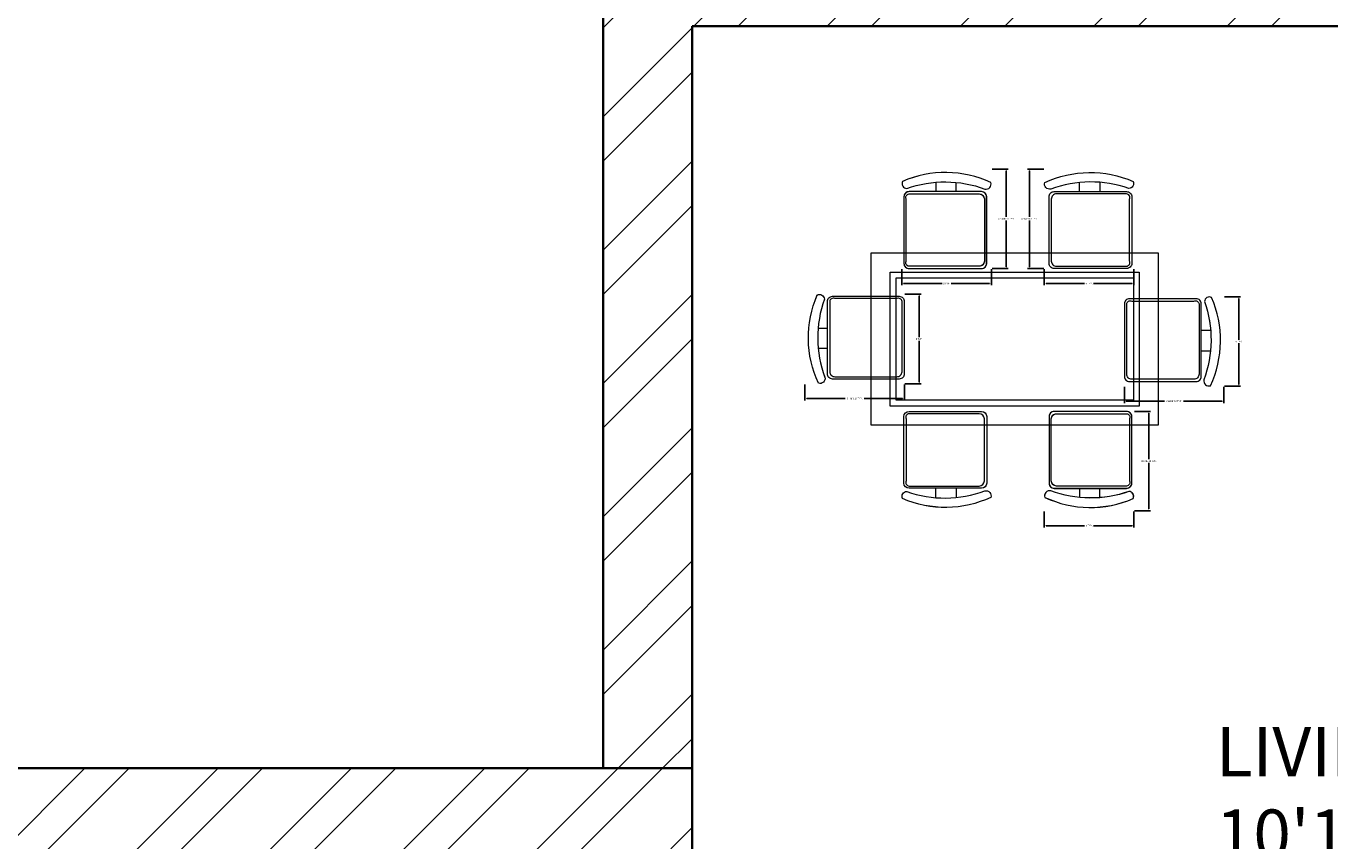
# Model space of a CAD drawing. Units: inches. Extents: x 2120 to 4013, y 1390 to 3019.
# Tile 37 of 59: x 2657 to 2789, y 2131 to 2213. Entities that reach past the tile are written whole.
import ezdxf

# ---------------------------------------------------------------- set-up
doc = ezdxf.new("R2010")
doc.units = ezdxf.units.IN
for name, color, linetype, lineweight in [('A-ANNO-DIMS', 2, 'Continuous', 18), ('A-AREA-IDEN', 7, 'Continuous', 18), ('A-FURN', 8, 'Continuous', 13), ('A-WALL', 7, 'Continuous', 35), ('A-WALL-PATT', 252, 'Continuous', 13)]:
    doc.layers.add(name, color=color, linetype=linetype, lineweight=lineweight)
doc.styles.get("Standard").update_dxf_attribs({"font": 'arial.ttf'})
doc.dimstyles.get("Standard").update_dxf_attribs({"dimtxt": 0.18, "dimasz": 0.18, "dimexe": 0.18, "dimexo": 0.0625, "dimgap": 0.09, "dimtad": 0, "dimtih": 1, "dimtoh": 1, "dimdec": 4, "dimzin": 0, "dimdsep": 46, "dimtxsty": 'Standard', "dimcen": 0.09, "dimadec": 0, "dimazin": 0, "dimtfac": 1, "dimtdec": 4, "dimtofl": 0, "dimtmove": 0, "dimatfit": 3, "dimfxl": 1, "dimtolj": 1, "dimtzin": 0, "dimarcsym": 0})

# ---------------------------------------------------------------- blocks, each defined once
blk = doc.blocks.new('TABLE-DINING')
for points in [[(0, 17.41), (29.01, 17.41), (29.01, 0), (0, 0)], [(1.93, 15.47), (27.08, 15.47), (27.08, 1.93), (1.93, 1.93)], [(2.51, 14.89), (26.5, 14.89), (26.5, 2.51), (2.51, 2.51)]]:
    blk.add_lwpolyline(points, close=True)
blk = doc.blocks.new('CHAIR-DINING-01')
for points in [[(1.68, 0.62, -0.578392), (1.02, 0.02, -0.214524), (0.9, 8.94, -0.552014), (1.62, 8.52, 0.175809), (1.68, 0.62)], [(1.93, 8.29, -0.414214), (2.45, 8.81), (9.19, 8.81, -0.414214), (9.7, 8.29), (9.7, 0.96, -0.414214), (9.19, 0.45), (2.45, 0.45, -0.414214), (1.93, 0.96), (1.93, 8.29)], [(1.93, 3.54), (1.01, 3.54, 0.064759)]]:
    blk.add_lwpolyline(points, format="xyb")
blk.add_lwpolyline([(2.16, 8.29), (2.16, 1.19, 0.414214), (2.68, 0.68), (8.96, 0.68, 0.414214), (9.47, 1.19), (9.47, 8.29, 0.512069), (8.96, 8.58), (2.68, 8.58, 0.512069)], format="xyb", close=True)
blk.add_lwpolyline([(0.99, 5.59), (1.93, 5.59)])
blk = doc.blocks.new('CHAIR-DINING-04')
for points in [[(7.77, 8.29, 0.414214), (7.26, 8.81), (0.51, 8.81, 0.414214), (0, 8.29), (0, 0.96, 0.414214), (0.51, 0.45), (7.26, 0.45, 0.414214), (7.77, 0.96), (7.77, 8.29)], [(8.09, 8.52, -0.175809), (8.03, 0.62, 0.578392), (8.69, 0.02, 0.214524), (8.81, 8.94, 0.552014), (8.09, 8.52, -0.065079)], [(7.77, 3.54), (8.7, 3.54, -0.064759)]]:
    blk.add_lwpolyline(points, format="xyb")
blk.add_lwpolyline([(7.54, 8.29), (7.54, 1.19, -0.414214), (7.03, 0.68), (0.74, 0.68, -0.414214), (0.23, 1.19), (0.23, 8.29, -0.512069), (0.74, 8.58), (7.03, 8.58, -0.512069)], format="xyb", close=True)
blk.add_lwpolyline([(8.72, 5.59), (7.77, 5.59)])
blk = doc.blocks.new('CHAIR-DINING-05')
for points in [[(1.68, 0.62, -0.578392), (1.02, 0.02, -0.214524), (0.9, 8.94, -0.552014), (1.62, 8.52, 0.175809), (1.68, 0.62)], [(1.93, 8.29, -0.414214), (2.45, 8.81), (9.19, 8.81, -0.414214), (9.7, 8.29), (9.7, 0.96, -0.414214), (9.19, 0.45), (2.45, 0.45, -0.414214), (1.93, 0.96), (1.93, 8.29)], [(1.93, 3.54), (1.01, 3.54, 0.064759)]]:
    blk.add_lwpolyline(points, format="xyb")
blk.add_lwpolyline([(2.16, 8.29), (2.16, 1.19, 0.414214), (2.68, 0.68), (8.96, 0.68, 0.414214), (9.47, 1.19), (9.47, 8.29, 0.512069), (8.96, 8.58), (2.68, 8.58, 0.512069)], format="xyb", close=True)
blk.add_lwpolyline([(0.99, 5.59), (1.93, 5.59)])
blk = doc.blocks.new('CHAIR-DINING-06')
for points in [[(7.77, 8.29, 0.414214), (7.26, 8.81), (0.51, 8.81, 0.414214), (0, 8.29), (0, 0.96, 0.414214), (0.51, 0.45), (7.26, 0.45, 0.414214), (7.77, 0.96), (7.77, 8.29)], [(8.09, 8.52, -0.175809), (8.03, 0.62, 0.578392), (8.69, 0.02, 0.214524), (8.81, 8.94, 0.552014), (8.09, 8.52, -0.065079)], [(7.77, 3.54), (8.7, 3.54, -0.064759)]]:
    blk.add_lwpolyline(points, format="xyb")
blk.add_lwpolyline([(7.54, 8.29), (7.54, 1.19, -0.414214), (7.03, 0.68), (0.74, 0.68, -0.414214), (0.23, 1.19), (0.23, 8.29, -0.512069), (0.74, 8.58), (7.03, 8.58, -0.512069)], format="xyb", close=True)
blk.add_lwpolyline([(8.72, 5.59), (7.77, 5.59)])
blk = doc.blocks.new('CHAIR-DINING-13')
for points in [[(0.47, 8.09, -0.175809), (8.38, 8.03, 0.578392), (8.97, 8.69, 0.214524), (0.06, 8.81, 0.552014), (0.47, 8.09, -0.065079)], [(5.46, 7.77), (5.46, 8.7, -0.064759)], [(8.04, 7.77), (0.71, 7.77, 0.414214), (0.19, 7.26), (0.19, 0.51, 0.414214), (0.71, 0), (8.04, 0, 0.414214), (8.55, 0.51), (8.55, 7.26, 0.414214), (8.04, 7.77)]]:
    blk.add_lwpolyline(points, format="xyb")
blk.add_lwpolyline([(3.41, 8.72), (3.41, 7.77)])
blk.add_lwpolyline([(0.71, 7.54), (7.81, 7.54, -0.414214), (8.32, 7.03), (8.32, 0.74, -0.414214), (7.81, 0.23), (0.71, 0.23, -0.512069), (0.42, 0.74), (0.42, 7.03, -0.512069)], format="xyb", close=True)
blk = doc.blocks.new('CHAIR-DINING-14')
for points in [[(1.68, 0.62, -0.578392), (1.02, 0.02, -0.214524), (0.9, 8.94, -0.552014), (1.62, 8.52, 0.175809), (1.68, 0.62)], [(1.93, 8.29, -0.414214), (2.45, 8.81), (9.19, 8.81, -0.414214), (9.7, 8.29), (9.7, 0.96, -0.414214), (9.19, 0.45), (2.45, 0.45, -0.414214), (1.93, 0.96), (1.93, 8.29)], [(1.93, 3.54), (1.01, 3.54, 0.064759)]]:
    blk.add_lwpolyline(points, format="xyb")
blk.add_lwpolyline([(2.16, 8.29), (2.16, 1.19, 0.414214), (2.68, 0.68), (8.96, 0.68, 0.414214), (9.47, 1.19), (9.47, 8.29, 0.512069), (8.96, 8.58), (2.68, 8.58, 0.512069)], format="xyb", close=True)
blk.add_lwpolyline([(0.99, 5.59), (1.93, 5.59)])
blk = doc.blocks.new('CHAIR-DINING-15')
for points in [[(8.29, 1.93, 0.414214), (8.81, 2.45), (8.81, 9.19, 0.414214), (8.29, 9.7), (0.96, 9.7, 0.414214), (0.45, 9.19), (0.45, 2.45, 0.414214), (0.96, 1.93), (8.29, 1.93)], [(8.52, 1.62, -0.175809), (0.62, 1.68, 0.578392), (0.02, 1.02, 0.214524), (8.94, 0.9, 0.552014), (8.52, 1.62, -0.065079)], [(3.54, 1.93), (3.54, 1.01, -0.064759)]]:
    blk.add_lwpolyline(points, format="xyb")
blk.add_lwpolyline([(8.29, 2.16), (1.19, 2.16, -0.414214), (0.68, 2.68), (0.68, 8.96, -0.414214), (1.19, 9.47), (8.29, 9.47, -0.512069), (8.58, 8.96), (8.58, 2.68, -0.512069)], format="xyb", close=True)
blk.add_lwpolyline([(5.59, 0.99), (5.59, 1.93)])
blk = doc.blocks.new('*D89')
at = {"layer": 'A-ANNO-DIMS', "color": 0, "lineweight": -2, "transparency": 16777216}
for p, q in [((2736.13, 2176.82), (2736.13, 2175.2)), ((2746.17, 2176.82), (2746.17, 2175.2)), ((2736.31, 2175.38), (2740.2, 2175.38)), ((2745.99, 2175.38), (2742.1, 2175.38))]:
    blk.add_line(p, q, dxfattribs=at)
at = {"layer": 'A-ANNO-DIMS', "color": 0, "transparency": 16777216}
for points in [[(2736.31, 2175.41), (2736.31, 2175.35), (2736.13, 2175.38)], [(2745.99, 2175.41), (2745.99, 2175.35), (2746.17, 2175.38)]]:
    blk.add_solid(points, dxfattribs=at)
at = {"layer": 'Defpoints', "color": 0, "transparency": 16777216}
for p in [(2736.13, 2176.88), (2746.17, 2176.88), (2746.17, 2175.38)]:
    blk.add_point(p, dxfattribs=at)
at = {"layer": 'A-ANNO-DIMS', "color": 0, "transparency": 16777216, "insert": (2741.15, 2175.38), "char_height": 0.18, "attachment_point": 5}
blk.add_mtext('\\A1;CHAIR 10 TYP.', dxfattribs=at)
blk = doc.blocks.new('*D90')
at = {"layer": 'A-ANNO-DIMS', "color": 0, "lineweight": -2, "transparency": 16777216}
for p, q in [((2746.23, 2185.94), (2747.86, 2185.94)), ((2747.68, 2185.76), (2747.68, 2181.59)), ((2747.68, 2177.06), (2747.68, 2181.23)), ((2746.23, 2176.88), (2747.86, 2176.88))]:
    blk.add_line(p, q, dxfattribs=at)
at = {"layer": 'A-ANNO-DIMS', "color": 0, "transparency": 16777216}
for points in [[(2747.65, 2185.76), (2747.71, 2185.76), (2747.68, 2185.94)], [(2747.65, 2177.06), (2747.71, 2177.06), (2747.68, 2176.88)]]:
    blk.add_solid(points, dxfattribs=at)
at = {"layer": 'Defpoints', "color": 0, "transparency": 16777216}
for p in [(2746.17, 2185.94), (2747.68, 2185.94), (2746.17, 2176.88)]:
    blk.add_point(p, dxfattribs=at)
at = {"layer": 'A-ANNO-DIMS', "color": 0, "transparency": 16777216, "insert": (2747.68, 2181.41), "char_height": 0.18, "attachment_point": 5}
blk.add_mtext('\\A1;9 TYP.', dxfattribs=at)
blk = doc.blocks.new('*D91')
at = {"layer": 'A-ANNO-DIMS', "color": 0, "lineweight": -2, "transparency": 16777216}
for p, q in [((2768.4, 2176.57), (2768.4, 2174.94)), ((2778.45, 2176.57), (2778.45, 2174.94)), ((2768.58, 2175.12), (2772.47, 2175.12)), ((2778.27, 2175.12), (2774.38, 2175.12))]:
    blk.add_line(p, q, dxfattribs=at)
at = {"layer": 'A-ANNO-DIMS', "color": 0, "transparency": 16777216}
for points in [[(2768.58, 2175.15), (2768.58, 2175.09), (2768.4, 2175.12)], [(2778.27, 2175.15), (2778.27, 2175.09), (2778.45, 2175.12)]]:
    blk.add_solid(points, dxfattribs=at)
at = {"layer": 'Defpoints', "color": 0, "transparency": 16777216}
for p in [(2768.4, 2176.63), (2778.45, 2176.63), (2778.45, 2175.12)]:
    blk.add_point(p, dxfattribs=at)
at = {"layer": 'A-ANNO-DIMS', "color": 0, "transparency": 16777216, "insert": (2773.43, 2175.12), "char_height": 0.18, "attachment_point": 5}
blk.add_mtext('\\A1;CHAIR 10 TYP.', dxfattribs=at)
blk = doc.blocks.new('*D92')
at = {"layer": 'A-ANNO-DIMS', "color": 0, "lineweight": -2, "transparency": 16777216}
for p, q in [((2778.51, 2185.68), (2780.14, 2185.68)), ((2779.96, 2185.5), (2779.96, 2181.34)), ((2779.96, 2176.81), (2779.96, 2180.98)), ((2778.51, 2176.63), (2780.14, 2176.63))]:
    blk.add_line(p, q, dxfattribs=at)
at = {"layer": 'A-ANNO-DIMS', "color": 0, "transparency": 16777216}
for points in [[(2779.93, 2185.5), (2779.99, 2185.5), (2779.96, 2185.68)], [(2779.93, 2176.81), (2779.99, 2176.81), (2779.96, 2176.63)]]:
    blk.add_solid(points, dxfattribs=at)
at = {"layer": 'Defpoints', "color": 0, "transparency": 16777216}
for p in [(2778.45, 2185.68), (2779.96, 2185.68), (2778.45, 2176.63)]:
    blk.add_point(p, dxfattribs=at)
at = {"layer": 'A-ANNO-DIMS', "color": 0, "transparency": 16777216, "insert": (2779.96, 2181.16), "char_height": 0.18, "attachment_point": 5}
blk.add_mtext('\\A1;9 TYP.', dxfattribs=at)
blk = doc.blocks.new('*D105')
at = {"layer": 'A-ANNO-DIMS', "color": 0, "lineweight": -2, "transparency": 16777216}
for p, q in [((2755.03, 2198.57), (2756.65, 2198.57)), ((2756.47, 2198.39), (2756.47, 2193.74)), ((2756.47, 2188.71), (2756.47, 2193.37)), ((2755.03, 2188.53), (2756.65, 2188.53))]:
    blk.add_line(p, q, dxfattribs=at)
at = {"layer": 'A-ANNO-DIMS', "color": 0, "transparency": 16777216}
for points in [[(2756.44, 2198.39), (2756.5, 2198.39), (2756.47, 2198.57)], [(2756.44, 2188.71), (2756.5, 2188.71), (2756.47, 2188.53)]]:
    blk.add_solid(points, dxfattribs=at)
at = {"layer": 'Defpoints', "color": 0, "transparency": 16777216}
for p in [(2754.97, 2198.57), (2756.47, 2198.57), (2754.97, 2188.53)]:
    blk.add_point(p, dxfattribs=at)
at = {"layer": 'A-ANNO-DIMS', "color": 0, "transparency": 16777216, "insert": (2756.47, 2193.55), "char_height": 0.18, "attachment_point": 5}
blk.add_mtext('\\A1;CHAIR 10 TYP.', dxfattribs=at)
blk = doc.blocks.new('*D106')
at = {"layer": 'A-ANNO-DIMS', "color": 0, "lineweight": -2, "transparency": 16777216}
for p, q in [((2745.91, 2188.47), (2745.91, 2186.84)), ((2754.97, 2188.47), (2754.97, 2186.84)), ((2746.09, 2187.02), (2749.98, 2187.02)), ((2754.79, 2187.02), (2750.9, 2187.02))]:
    blk.add_line(p, q, dxfattribs=at)
at = {"layer": 'A-ANNO-DIMS', "color": 0, "transparency": 16777216}
for points in [[(2746.09, 2187.05), (2746.09, 2186.99), (2745.91, 2187.02)], [(2754.79, 2187.05), (2754.79, 2186.99), (2754.97, 2187.02)]]:
    blk.add_solid(points, dxfattribs=at)
at = {"layer": 'Defpoints', "color": 0, "transparency": 16777216}
for p in [(2745.91, 2188.53), (2754.97, 2188.53), (2754.97, 2187.02)]:
    blk.add_point(p, dxfattribs=at)
at = {"layer": 'A-ANNO-DIMS', "color": 0, "transparency": 16777216, "insert": (2750.44, 2187.02), "char_height": 0.18, "attachment_point": 5}
blk.add_mtext('\\A1;9 TYP.', dxfattribs=at)
blk = doc.blocks.new('*D107')
at = {"layer": 'A-ANNO-DIMS', "color": 0, "lineweight": -2, "transparency": 16777216}
for p, q in [((2760.25, 2198.57), (2758.62, 2198.57)), ((2758.8, 2198.39), (2758.8, 2193.74)), ((2758.8, 2188.71), (2758.8, 2193.37)), ((2760.25, 2188.53), (2758.62, 2188.53))]:
    blk.add_line(p, q, dxfattribs=at)
at = {"layer": 'A-ANNO-DIMS', "color": 0, "transparency": 16777216}
for points in [[(2758.77, 2198.39), (2758.83, 2198.39), (2758.8, 2198.57)], [(2758.77, 2188.71), (2758.83, 2188.71), (2758.8, 2188.53)]]:
    blk.add_solid(points, dxfattribs=at)
at = {"layer": 'Defpoints', "color": 0, "transparency": 16777216}
for p in [(2760.31, 2198.57), (2758.8, 2188.53), (2760.31, 2188.53)]:
    blk.add_point(p, dxfattribs=at)
at = {"layer": 'A-ANNO-DIMS', "color": 0, "transparency": 16777216, "insert": (2758.8, 2193.55), "char_height": 0.18, "attachment_point": 5}
blk.add_mtext('\\A1;CHAIR 10 TYP.', dxfattribs=at)
blk = doc.blocks.new('*D108')
at = {"layer": 'A-ANNO-DIMS', "color": 0, "lineweight": -2, "transparency": 16777216}
for p, q in [((2760.31, 2188.47), (2760.31, 2186.84)), ((2769.36, 2188.47), (2769.36, 2186.84)), ((2760.49, 2187.02), (2764.38, 2187.02)), ((2769.18, 2187.02), (2765.29, 2187.02))]:
    blk.add_line(p, q, dxfattribs=at)
at = {"layer": 'A-ANNO-DIMS', "color": 0, "transparency": 16777216}
for points in [[(2760.49, 2187.05), (2760.49, 2186.99), (2760.31, 2187.02)], [(2769.18, 2187.05), (2769.18, 2186.99), (2769.36, 2187.02)]]:
    blk.add_solid(points, dxfattribs=at)
at = {"layer": 'Defpoints', "color": 0, "transparency": 16777216}
for p in [(2760.31, 2188.53), (2769.36, 2188.53), (2769.36, 2187.02)]:
    blk.add_point(p, dxfattribs=at)
at = {"layer": 'A-ANNO-DIMS', "color": 0, "transparency": 16777216, "insert": (2764.84, 2187.02), "char_height": 0.18, "attachment_point": 5}
blk.add_mtext('\\A1;9 TYP.', dxfattribs=at)
blk = doc.blocks.new('*D109')
at = {"layer": 'A-ANNO-DIMS', "color": 0, "lineweight": -2, "transparency": 16777216}
for p, q in [((2769.43, 2174.09), (2771.05, 2174.09)), ((2770.87, 2173.91), (2770.87, 2169.25)), ((2770.87, 2164.23), (2770.87, 2168.89)), ((2769.43, 2164.05), (2771.05, 2164.05))]:
    blk.add_line(p, q, dxfattribs=at)
at = {"layer": 'A-ANNO-DIMS', "color": 0, "transparency": 16777216}
for points in [[(2770.84, 2173.91), (2770.9, 2173.91), (2770.87, 2174.09)], [(2770.84, 2164.23), (2770.9, 2164.23), (2770.87, 2164.05)]]:
    blk.add_solid(points, dxfattribs=at)
at = {"layer": 'Defpoints', "color": 0, "transparency": 16777216}
for p in [(2769.36, 2174.09), (2770.87, 2174.09), (2769.36, 2164.05)]:
    blk.add_point(p, dxfattribs=at)
at = {"layer": 'A-ANNO-DIMS', "color": 0, "transparency": 16777216, "insert": (2770.87, 2169.07), "char_height": 0.18, "attachment_point": 5}
blk.add_mtext('\\A1;CHAIR 10 TYP.', dxfattribs=at)
blk = doc.blocks.new('*D110')
at = {"layer": 'A-ANNO-DIMS', "color": 0, "lineweight": -2, "transparency": 16777216}
for p, q in [((2760.31, 2163.98), (2760.31, 2162.36)), ((2769.36, 2163.98), (2769.36, 2162.36)), ((2760.49, 2162.54), (2764.38, 2162.54)), ((2769.18, 2162.54), (2765.29, 2162.54))]:
    blk.add_line(p, q, dxfattribs=at)
at = {"layer": 'A-ANNO-DIMS', "color": 0, "transparency": 16777216}
for points in [[(2760.49, 2162.57), (2760.49, 2162.51), (2760.31, 2162.54)], [(2769.18, 2162.57), (2769.18, 2162.51), (2769.36, 2162.54)]]:
    blk.add_solid(points, dxfattribs=at)
at = {"layer": 'Defpoints', "color": 0, "transparency": 16777216}
for p in [(2760.31, 2164.05), (2769.36, 2164.05), (2769.36, 2162.54)]:
    blk.add_point(p, dxfattribs=at)
at = {"layer": 'A-ANNO-DIMS', "color": 0, "transparency": 16777216, "insert": (2764.84, 2162.54), "char_height": 0.18, "attachment_point": 5}
blk.add_mtext('\\A1;9 TYP.', dxfattribs=at)

msp = doc.modelspace()

# ---------------------------------------------------------------- hatches: boundary and pattern name
at = {"layer": 'A-WALL-PATT'}
h = msp.add_hatch(dxfattribs=at)
h.set_pattern_fill('ANSI32', color=256)
h.paths.add_polyline_path([(2271.7331, 2122.6377), (2262.7331, 2122.6377), (2262.7331, 2040.3893), (2267.2331, 2040.3893), (2271.7331, 2040.3893), (2271.7331, 2044.8856), (2271.7331, 2070.531), (2391.7331, 2070.531), (2391.7331, 1926.5306), (2388.3993, 1926.5306), (2388.3993, 1922.531), (2395.7331, 1922.531), (2395.7331, 1992.531), (2400.4511, 1992.531), (2400.4511, 1997.0306), (2395.7331, 1997.0306), (2395.7331, 2070.531), (2443.7331, 2070.531), (2443.7331, 2046.1368), (2448.2331, 2046.1368), (2448.2331, 2070.531), (2580.2331, 2070.531), (2580.2331, 1997.0306), (2492.9076, 1997.0306), (2492.9076, 1992.531), (2580.2331, 1992.531), (2580.2331, 1983.9368), (2589.2331, 1983.9368), (2589.2331, 2070.531), (2589.2331, 2075.0306), (2396.2331, 2075.0306), (2396.2331, 2184.3565), (2393.9831, 2184.3565), (2391.7331, 2184.3565), (2391.7331, 2075.0306), (2271.7331, 2075.0306)])
h.paths.add_polyline_path([(2724.7331, 2138.0306), (2628.7331, 2138.0306), (2628.7331, 2070.5306), (2628.7331, 2067.0987), (2633.2331, 2067.0987), (2637.7331, 2067.0987), (2637.7331, 2070.531), (2657.3413, 2070.531), (2657.3413, 2079.5306), (2637.7331, 2079.5306), (2637.7331, 2129.031), (2715.7331, 2129.031), (2715.7331, 2079.5306), (2698.0378, 2079.5306), (2698.0378, 2070.531), (2715.7331, 2070.531), (2715.7331, 2012.1531), (2720.2331, 2012.1531), (2724.7331, 2012.1531)])
h.paths.add_polyline_path([(2724.7331, 2213.031), (2831.3209, 2213.031), (2831.3209, 2215.281), (2831.3209, 2217.5306), (2724.7331, 2217.5306), (2724.7331, 2343.531), (2751.8755, 2343.531), (2751.8755, 2352.5306), (2715.7331, 2352.5306), (2715.7331, 2138.031), (2724.7331, 2138.031)])
h.paths.add_polyline_path([(2902.53, 2352.5306), (2811.8755, 2352.5306), (2811.8755, 2343.531), (2867.2331, 2343.531), (2867.2331, 2217.5306), (2863.6364, 2217.5306), (2863.6364, 2213.031), (2871.7331, 2213.031), (2871.7331, 2217.531), (2871.7331, 2343.531), (2902.53, 2343.531)])
h.paths.add_polyline_path([(3009.7331, 2352.5306), (2938.53, 2352.5306), (2938.53, 2343.531), (2966.2331, 2343.531), (2966.2331, 2242.3281), (2968.4831, 2242.3281), (2970.7331, 2242.3281), (2970.7331, 2343.531), (3009.7331, 2343.531)])
h.paths.add_polyline_path([(3009.7331, 2217.5306), (2970.7331, 2217.5306), (2970.7331, 2220.5422), (2968.4831, 2220.5422), (2966.2331, 2220.5422), (2966.2331, 2217.5306), (2911.7752, 2217.5306), (2907.7331, 2217.5306), (2907.7331, 2213.0306), (2907.7331, 2194.9663), (2912.2331, 2194.9663), (2912.2331, 2213.031), (2970.7331, 2213.031), (3000.7331, 2213.031), (3000.7331, 2205.523), (3009.7331, 2205.523)])
h.paths.add_polyline_path([(3009.7331, 2181.5227), (3000.7331, 2181.5227), (3000.7331, 2165.0306), (2912.2331, 2165.0306), (2912.2331, 2170.8202), (2907.7331, 2170.8202), (2907.7331, 2165.0306), (2899.5169, 2165.0306), (2899.5169, 2162.7806), (2899.5169, 2160.531), (2907.7331, 2160.531), (2907.7331, 2137.3432), (2912.2331, 2137.3432), (2912.2331, 2160.531), (3000.7331, 2160.531), (3000.7331, 2150.4993), (3009.7331, 2150.4993)])
h.paths.add_polyline_path([(3009.7331, 2126.499), (3005.2331, 2126.499), (3000.7331, 2126.499), (3000.7331, 2112.5306), (2912.2331, 2112.5306), (2912.2331, 2115.6036), (2907.7331, 2115.6036), (2907.7331, 2108.031), (3000.7331, 2108.031), (3000.7331, 2084.7256), (3009.7331, 2084.7256)], flags=17)
h.paths.add_polyline_path([(3009.7331, 1971.531), (3009.7331, 2024.7253), (3000.7331, 2024.7253), (3000.7331, 2006.4153), (3000.7331, 1971.5306), (2864.2331, 1971.5306), (2864.2331, 2160.531), (2868.0522, 2160.531), (2868.0522, 2165.0306), (2859.7331, 2165.0306), (2859.7331, 1971.5306), (2724.7331, 1971.5306), (2724.7331, 1977.7012), (2715.7331, 1977.7012), (2715.7331, 1962.5306), (2715.7331, 1950.9035), (2720.2331, 1950.9035), (2724.7331, 1950.9035), (2724.7331, 1962.531), (2855.2331, 1962.531), (2859.7331, 1962.531), (2859.7331, 1835.031), (2864.2331, 1834.8158), (2864.2331, 1962.531), (2958.7331, 1962.531), (2958.7331, 1937.0925), (2963.2331, 1937.0925), (2963.2331, 1962.531), (3000.7331, 1962.531), (3009.7331, 1962.531)])
h.paths.add_polyline_path([(2724.7331, 1728.531), (2822.7164, 1728.531), (2822.7164, 1733.0306), (2724.7331, 1733.0306), (2724.7331, 1779.3416), (2715.7331, 1779.3416), (2715.7331, 1581.531), (2753.02, 1581.531), (2753.02, 1586.031), (2753.02, 1590.5306), (2724.7331, 1590.5306)])
h.paths.add_polyline_path([(2864.2331, 1590.531), (2864.2331, 1787.031), (2868.4075, 1787.031), (2868.4075, 1791.5306), (2859.7331, 1791.5306), (2859.7331, 1739.0306), (2859.7331, 1733.0306), (2854.3125, 1733.0306), (2854.3125, 1728.531), (2859.7331, 1728.531), (2859.7331, 1590.5306), (2813.02, 1590.5306), (2813.02, 1581.531), (2868.4123, 1581.531), (2868.4123, 1583.781), (2868.4123, 1586.0306), (2864.2331, 1586.0306)])
h.paths.add_polyline_path([(3009.7331, 1754.6619), (3000.7331, 1754.6619), (3000.7331, 1739.0306), (2912.2331, 1739.0306), (2912.2331, 1742.2257), (2907.7331, 1742.2257), (2907.7331, 1739.0306), (2907.7331, 1734.531), (3000.7331, 1734.531), (3000.7331, 1590.5306), (3000.7331, 1586.0306), (2971.3921, 1586.0306), (2971.3921, 1581.531), (3009.7331, 1581.531)])
h.paths.add_polyline_path([(2911.3921, 1583.781), (2911.3921, 1586.0306), (2891.2138, 1586.0306), (2891.2138, 1581.531), (2911.3921, 1581.531)])
h.paths.add_polyline_path([(3009.7331, 1799.8422), (3000.7331, 1799.8422), (3000.7331, 1791.5306), (2912.2331, 1791.5306), (2912.2331, 1796.3264), (2909.9831, 1796.3264), (2907.7331, 1796.3264), (2907.7331, 1791.5306), (2902.7033, 1791.5306), (2902.7033, 1787.031), (2907.7331, 1787.031), (2907.7331, 1761.1622), (2912.2331, 1761.1622), (2912.2331, 1787.031), (3000.7331, 1787.031), (3000.7331, 1778.6622), (3009.7331, 1778.6622)])
h.paths.add_polyline_path([(3009.7331, 1839.5306), (2963.2331, 1839.5306), (2963.2331, 1842.8629), (2960.9831, 1842.8629), (2958.7331, 1842.8629), (2958.7331, 1839.5306), (2907.7331, 1839.5306), (2907.7331, 1814.4599), (2912.2331, 1814.4599), (2912.2331, 1835.031), (3000.7331, 1835.031), (3000.7331, 1823.8425), (3009.7331, 1823.8425), (3009.7331, 1835.031)])
h.paths.add_polyline_path([(2963.2331, 1901.0922), (2960.9831, 1901.0922), (2958.7331, 1901.0922), (2958.7331, 1862.8843), (2963.2331, 1862.8843)], flags=17)
h.paths.add_polyline_path([(2724.7331, 1891.9826), (2724.7331, 1914.3416), (2715.7331, 1914.3416), (2715.7331, 1783.8416), (2637.7331, 1783.8416), (2637.7331, 1914.3416), (2628.7331, 1914.3416), (2624.7701, 1914.3416), (2624.7701, 1909.8416), (2624.7701, 1905.3419), (2628.7331, 1905.3419), (2628.7331, 1876.9915), (2628.7331, 1779.3419), (2637.7331, 1779.3419), (2715.7331, 1779.3419), (2724.7331, 1779.3419), (2724.7331, 1835.031)])
h.paths.add_polyline_path([(2637.7331, 1731.531), (2637.7331, 1779.3416), (2628.7331, 1779.3416), (2628.7331, 1731.5306), (2589.2331, 1731.5306), (2535.9814, 1731.5306), (2496.7331, 1731.5306), (2496.7331, 1725.6876), (2498.9831, 1725.6876), (2501.2331, 1725.6876), (2501.2331, 1727.031), (2628.7331, 1727.031), (2628.7331, 1680.4203), (2628.7331, 1590.5306), (2628.7331, 1586.0306), (2604.1361, 1586.0306), (2604.1361, 1581.531), (2637.7331, 1581.531), (2637.7331, 1590.531)])

# ---------------------------------------------------------------- linework, layer by layer
at = {"layer": 'A-FURN'}
for points in [[(2746.4103, 2196.6188, -0.17580919), (2754.312, 2196.559, 0.57839206), (2754.9106, 2197.2172, 0.21452438), (2745.9913, 2197.3369, 0.55201397), (2746.4103, 2196.6188, -0.06507904)], [(2753.9768, 2196.3017), (2746.6411, 2196.3017, 0.41421356), (2746.1279, 2195.7884), (2746.1279, 2189.0434, 0.41421356), (2746.6411, 2188.5302), (2753.9768, 2188.5302, 0.41421356), (2754.49, 2189.0434), (2754.49, 2195.7884, 0.41421356), (2753.9768, 2196.3017)], [(2751.4001, 2196.3017), (2751.4001, 2197.2294, -0.06475861)], [(2753.9767, 2166.3187), (2746.6411, 2166.3187, -0.41421356), (2746.1279, 2166.8319), (2746.1279, 2173.577, -0.41421356), (2746.6411, 2174.0902), (2753.9767, 2174.0902, -0.41421356), (2754.49, 2173.577), (2754.49, 2166.8319, -0.41421356), (2753.9767, 2166.3187)], [(2753.9768, 2166.3184), (2746.6411, 2166.3184, -0.41421356), (2746.1279, 2166.8316), (2746.1279, 2173.5767, -0.41421356), (2746.6411, 2174.0899), (2753.9768, 2174.0899, -0.41421356), (2754.49, 2173.5767), (2754.49, 2166.8316, -0.41421356), (2753.9768, 2166.3184)], [(2768.6351, 2166.3184, 0.41421356), (2769.1483, 2166.8316), (2769.1483, 2173.5767, 0.41421356), (2768.6351, 2174.0899), (2761.2994, 2174.0899, 0.41421356), (2760.7862, 2173.5767), (2760.7862, 2166.8316, 0.41421356), (2761.2994, 2166.3184), (2768.6351, 2166.3184)], [(2754.312, 2166.0614, -0.57839206), (2754.9106, 2165.4032, -0.21452438), (2745.9912, 2165.2835, -0.55201397), (2746.4103, 2166.0016, 0.17580929), (2754.312, 2166.0614)], [(2754.312, 2166.0611, -0.57839206), (2754.9106, 2165.4029, -0.21452438), (2745.9913, 2165.2832, -0.55201397), (2746.4103, 2166.0013, 0.17580929), (2754.312, 2166.0611)], [(2751.4001, 2166.3187), (2751.4001, 2165.391, 0.06475861)], [(2751.4001, 2166.3184), (2751.4001, 2165.3907, 0.06475861)], [(2768.8659, 2166.0013, -0.17580928), (2760.9642, 2166.0611, 0.57839206), (2760.3656, 2165.4029, 0.21452438), (2769.2849, 2165.2832, 0.55201397), (2768.8659, 2166.0013, -0.06507904)], [(2763.8761, 2166.3184), (2763.8761, 2165.3907, -0.06475861)]]:
    msp.add_lwpolyline(points, format="xyb", dxfattribs=at)
for points in [[(2746.6442, 2196.0704), (2753.7456, 2196.0704, -0.41421356), (2754.2588, 2195.5572), (2754.2588, 2189.2746, -0.41421356), (2753.7456, 2188.7614), (2746.6442, 2188.7614, -0.51206948), (2746.3591, 2189.2746), (2746.3591, 2195.5572, -0.51206948)], [(2746.6442, 2166.5499), (2753.7455, 2166.5499, 0.41421356), (2754.2587, 2167.0632), (2754.2587, 2173.3458, 0.41421356), (2753.7455, 2173.859), (2746.6442, 2173.859, 0.51206948), (2746.3591, 2173.3458), (2746.3591, 2167.0632, 0.51206948)], [(2746.6442, 2166.5496), (2753.7456, 2166.5496, 0.41421356), (2754.2588, 2167.0628), (2754.2588, 2173.3455, 0.41421356), (2753.7456, 2173.8587), (2746.6442, 2173.8587, 0.51206948), (2746.3591, 2173.3455), (2746.3591, 2167.0628, 0.51206948)], [(2768.632, 2166.5496), (2761.5306, 2166.5496, -0.41421356), (2761.0174, 2167.0628), (2761.0174, 2173.3455, -0.41421356), (2761.5306, 2173.8587), (2768.632, 2173.8587, -0.51206948), (2768.9171, 2173.3455), (2768.9171, 2167.0628, -0.51206948)]]:
    msp.add_lwpolyline(points, format="xyb", close=True, dxfattribs=at)
for points in [[(2749.3467, 2197.2463), (2749.3467, 2196.3017)], [(2749.3467, 2165.3741), (2749.3467, 2166.3187)], [(2749.3467, 2165.3738), (2749.3467, 2166.3184)], [(2765.9295, 2165.3738), (2765.9295, 2166.3184)]]:
    msp.add_lwpolyline(points, dxfattribs=at)
at = {"layer": 'A-WALL'}
for p, q in [((2715.7331, 2352.531), (2715.7331, 2138.031)), ((2715.7331, 2352.5306), (2715.7331, 2138.0306)), ((2724.7331, 2138.031), (2724.7331, 2213.031)), ((2724.7331, 2213.031), (2724.7331, 2010.5745)), ((2724.7331, 2138.0306), (2724.7331, 2213.0306)), ((2831.3209, 2213.0306), (2724.7331, 2213.0306)), ((2724.7331, 2213.0306), (2724.7331, 2010.5742)), ((2724.7331, 2138.031), (2628.7331, 2138.031)), ((2724.7331, 2138.0306), (2628.7331, 2138.0306)), ((2724.7331, 2129.031), (2724.7331, 2138.031)), ((2724.7331, 2129.0306), (2724.7331, 2138.0306))]:
    msp.add_line(p, q, dxfattribs=at)

# ---------------------------------------------------------------- block references
at = {"layer": 'A-FURN'}
for name, p in [('CHAIR-DINING-13', (2745.9356, 2188.5305)), ('TABLE-DINING', (2742.8219, 2172.7003)), ('TABLE-DINING', (2742.822, 2172.7)), ('CHAIR-DINING-14', (2736.4678, 2176.9145)), ('CHAIR-DINING-05', (2736.4678, 2176.9142)), ('CHAIR-DINING-04', (2768.4047, 2176.6632)), ('CHAIR-DINING-06', (2768.4047, 2176.6629)), ('CHAIR-DINING-15', (2760.341, 2164.3857))]:
    msp.add_blockref(name, p, dxfattribs=at)
for name, p, rotation in [('CHAIR-DINING-01', (2760.341, 2198.235), 269.999998092181), ('CHAIR-DINING-14', (2760.341, 2198.2347), 269.9999980921654)]:
    msp.add_blockref(name, p, dxfattribs=dict(at, rotation=rotation))

# ---------------------------------------------------------------- texts
at = {"layer": 'A-AREA-IDEN', "insert": (2777.6505, 2142.1991), "char_height": 5, "attachment_point": 1}
msp.add_mtext_dynamic_manual_height_columns('LIVING\\\\DINING\\P10\'10.5"X20\'1.5"', width=185.907328, gutter_width=12.5, heights=[0], dxfattribs=at)

# ---------------------------------------------------------------- dimensions: what is measured, and where the dimension line sits
at = {"layer": 'A-ANNO-DIMS'}
for base, p1, p2, angle, text, picture, middle in [((2756.4734, 2198.5747), (2754.9667, 2188.5305), (2754.9667, 2198.5747), 90, 'CHAIR <> TYP.', '*D105', (2756.4734, 2193.5526)), ((2758.8028, 2188.5302), (2760.3094, 2198.5744), (2760.3094, 2188.5302), 269.999998, 'CHAIR <> TYP.', '*D107', (2758.8028, 2193.5523)), ((2769.363, 2187.0236), (2760.3094, 2188.5302), (2769.363, 2188.5302), 359.999998, '<> TYP.', '*D108', (2764.8362, 2187.0236)), ((2747.679, 2185.9361), (2746.1723, 2176.8826), (2746.1723, 2185.9361), 90, '<> TYP.', '*D90', (2747.679, 2181.4094)), ((2779.9556, 2185.6849), (2778.4489, 2176.6314), (2778.4489, 2185.6849), 90, '<> TYP.', '*D92', (2779.9556, 2181.1581)), ((2770.8696, 2174.0902), (2769.3629, 2164.046), (2769.3629, 2174.0902), 90, 'CHAIR <> TYP.', '*D109', (2770.8696, 2169.0681))]:
    dim = msp.add_linear_dim(base=base, p1=p1, p2=p2, angle=angle, text=text, dimstyle='Standard', override={"dimdec": 0, "dimlfac": 1, "dimrnd": 0, "dimzin": 0, "dimdsep": 46, "dimlunit": 2}, dxfattribs=at)
    dim.commit()
    dim.dimension.update_dxf_attribs({"geometry": picture, "text_midpoint": middle})
for base, p1, p2, text, picture, middle in [((2754.9667, 2187.0239), (2745.9132, 2188.5305), (2754.9667, 2188.5305), '<> TYP.', '*D106', (2750.44, 2187.0239)), ((2746.1723, 2175.376), (2736.1281, 2176.8826), (2746.1723, 2176.8826), 'CHAIR <> TYP.', '*D89', (2741.1502, 2175.376)), ((2778.4489, 2175.1248), (2768.4047, 2176.6314), (2778.4489, 2176.6314), 'CHAIR <> TYP.', '*D91', (2773.4268, 2175.1248)), ((2769.3629, 2162.5394), (2760.3094, 2164.046), (2769.3629, 2164.046), '<> TYP.', '*D110', (2764.8362, 2162.5394))]:
    dim = msp.add_linear_dim(base=base, p1=p1, p2=p2, text=text, dimstyle='Standard', override={"dimdec": 0, "dimlfac": 1, "dimrnd": 0, "dimzin": 0, "dimdsep": 46, "dimlunit": 2}, dxfattribs=at)
    dim.commit()
    dim.dimension.update_dxf_attribs({"geometry": picture, "text_midpoint": middle})

doc.saveas('drawing.dxf')
